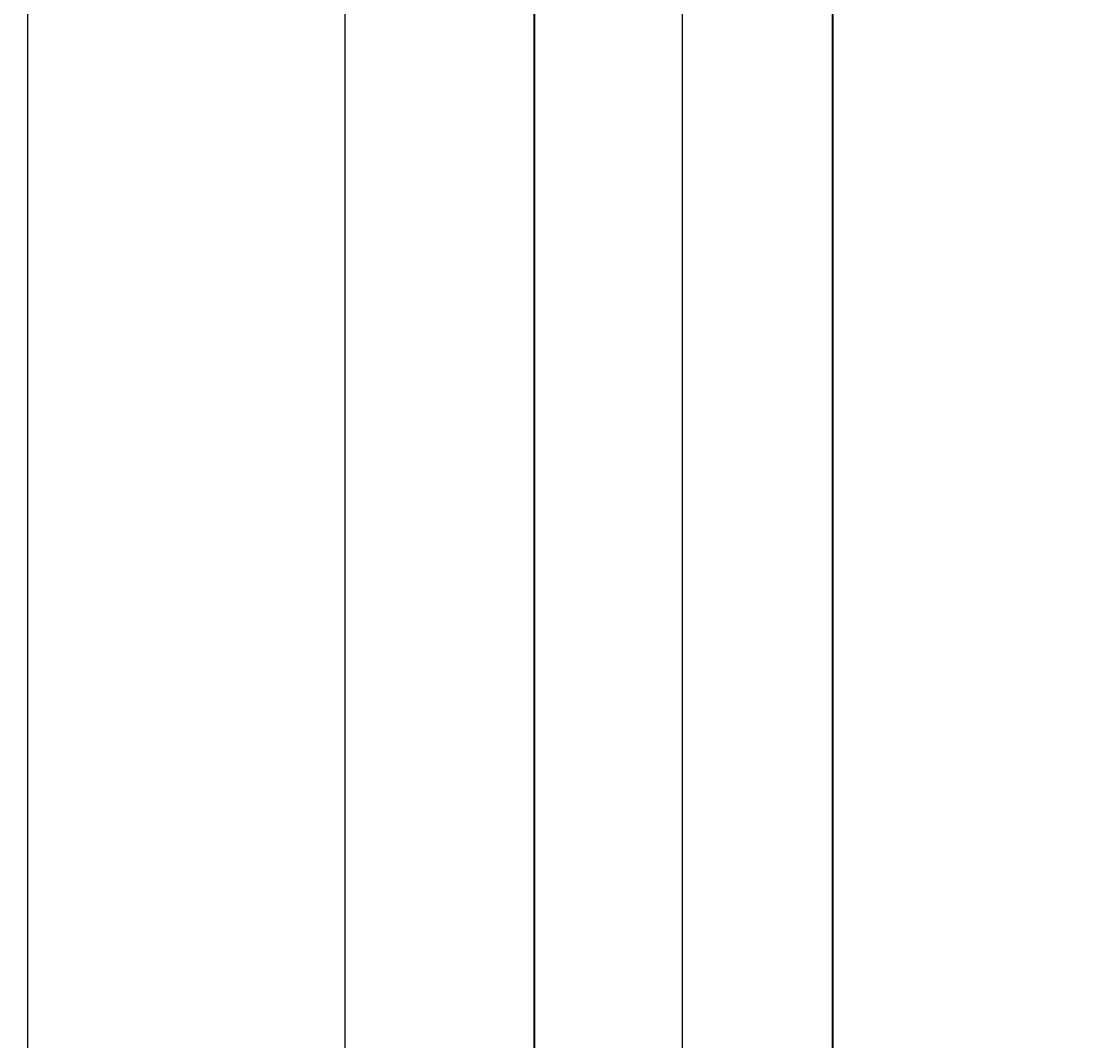
# Model space of a CAD drawing. Units: inches. Extents: x -6 to 289, y -8 to 323.
# Tile 43 of 107: x -6 to 46, y 223 to 273. Entities that reach past the tile are written whole.
import ezdxf

# ---------------------------------------------------------------- set-up
doc = ezdxf.new("R2010")
doc.units = ezdxf.units.IN
doc.header["$MEASUREMENT"] = 0
doc.layers.add('A-ANNO-DIMS', color=2, linetype='Continuous', lineweight=18)
doc.layers.add('A-ELEV', color=7, linetype='Continuous', lineweight=35)
doc.styles.get("Standard").update_dxf_attribs({"font": 'arial.ttf'})
doc.dimstyles.get("Standard").update_dxf_attribs({"dimtxt": 0.18, "dimasz": 0.18, "dimexe": 0.18, "dimexo": 0.0625, "dimgap": 0.09, "dimtad": 0, "dimtih": 1, "dimtoh": 1, "dimdec": 4, "dimzin": 0, "dimdsep": 46, "dimtxsty": 'Standard', "dimcen": 0.09, "dimadec": 0, "dimazin": 0, "dimtfac": 1, "dimtdec": 4, "dimtofl": 0, "dimtmove": 0, "dimatfit": 3, "dimfxl": 1, "dimtolj": 1, "dimtzin": 0, "dimarcsym": 0})

# ---------------------------------------------------------------- blocks, each defined once
blk = doc.blocks.new('*D19')
at = {"layer": 'A-ANNO-DIMS', "color": 0, "lineweight": -2, "transparency": 16777216}
for p, q in [((45.681, 277.043), (-5.737, 277.043)), ((-5.557, 276.863), (-5.557, 179.825)), ((-5.557, 82.423), (-5.557, 179.461)), ((45.681, 82.243), (-5.737, 82.243))]:
    blk.add_line(p, q, dxfattribs=at)
at = {"layer": 'A-ANNO-DIMS', "color": 0, "transparency": 16777216}
for points in [[(-5.587, 276.863), (-5.527, 276.863), (-5.557, 277.043)], [(-5.587, 82.423), (-5.527, 82.423), (-5.557, 82.243)]]:
    blk.add_solid(points, dxfattribs=at)
at = {"layer": 'Defpoints', "color": 0, "transparency": 16777216}
for p in [(-5.557, 277.043), (45.744, 277.043), (45.744, 82.243)]:
    blk.add_point(p, dxfattribs=at)
at = {"layer": 'A-ANNO-DIMS', "color": 0, "transparency": 16777216, "insert": (-5.557, 179.643), "char_height": 0.18, "attachment_point": 5}
blk.add_mtext('\\A1;194.8', dxfattribs=at)
blk = doc.blocks.new('*D22')
at = {"layer": 'A-ANNO-DIMS', "color": 0, "lineweight": -2, "transparency": 16777216}
for p, q in [((19.101, 307.289), (-5.737, 307.289)), ((-5.557, 307.109), (-5.557, 157.471)), ((-5.557, 7.469), (-5.557, 157.107)), ((11.907, 7.289), (-5.737, 7.289))]:
    blk.add_line(p, q, dxfattribs=at)
at = {"layer": 'A-ANNO-DIMS', "color": 0, "transparency": 16777216}
for points in [[(-5.587, 307.109), (-5.527, 307.109), (-5.557, 307.289)], [(-5.587, 7.469), (-5.527, 7.469), (-5.557, 7.289)]]:
    blk.add_solid(points, dxfattribs=at)
at = {"layer": 'Defpoints', "color": 0, "transparency": 16777216}
for p in [(19.164, 307.289), (-5.557, 7.289), (11.969, 7.289)]:
    blk.add_point(p, dxfattribs=at)
at = {"layer": 'A-ANNO-DIMS', "color": 0, "transparency": 16777216, "insert": (-5.557, 157.289), "char_height": 0.18, "attachment_point": 5}
blk.add_mtext('\\A1;300', dxfattribs=at)
blk = doc.blocks.new('*D27')
at = {"layer": 'A-ANNO-DIMS', "color": 0, "lineweight": -2, "transparency": 16777216}
for p, q in [((19.226, 307.289), (288.653, 307.289)), ((288.473, 307.109), (288.473, 277.471)), ((288.473, 247.469), (288.473, 277.107)), ((247.226, 247.289), (288.653, 247.289))]:
    blk.add_line(p, q, dxfattribs=at)
at = {"layer": 'A-ANNO-DIMS', "color": 0, "transparency": 16777216}
for points in [[(288.443, 307.109), (288.503, 307.109), (288.473, 307.289)], [(288.443, 247.469), (288.503, 247.469), (288.473, 247.289)]]:
    blk.add_solid(points, dxfattribs=at)
at = {"layer": 'Defpoints', "color": 0, "transparency": 16777216}
for p in [(19.164, 307.289), (288.473, 307.289), (247.164, 247.289)]:
    blk.add_point(p, dxfattribs=at)
at = {"layer": 'A-ANNO-DIMS', "color": 0, "transparency": 16777216, "insert": (288.473, 277.289), "char_height": 0.18, "attachment_point": 5}
blk.add_mtext('\\A1;60', dxfattribs=at)
blk = doc.blocks.new('*D57')
at = {"layer": 'A-ANNO-DIMS', "color": 0, "lineweight": -2, "transparency": 16777216}
for p, q in [((9.943, 68.495), (9.943, 322.969)), ((10.123, 322.789), (17.788, 322.789)), ((26.223, 322.789), (18.558, 322.789)), ((26.403, 68.495), (26.403, 322.969))]:
    blk.add_line(p, q, dxfattribs=at)
at = {"layer": 'A-ANNO-DIMS', "color": 0, "transparency": 16777216}
for points in [[(10.123, 322.819), (10.123, 322.759), (9.943, 322.789)], [(26.223, 322.819), (26.223, 322.759), (26.403, 322.789)]]:
    blk.add_solid(points, dxfattribs=at)
at = {"layer": 'Defpoints', "color": 0, "transparency": 16777216}
for p in [(26.403, 322.789), (9.943, 68.432), (26.403, 68.432)]:
    blk.add_point(p, dxfattribs=at)
at = {"layer": 'A-ANNO-DIMS', "color": 0, "transparency": 16777216, "insert": (18.173, 322.789), "char_height": 0.18, "attachment_point": 5}
blk.add_mtext('\\A1;16.46', dxfattribs=at)

msp = doc.modelspace()

# ---------------------------------------------------------------- linework, layer by layer
at = {"layer": 'A-ELEV'}
msp.add_line((19.1638, 307.2888), (19.1638, 68.4322), dxfattribs=at)
msp.add_lwpolyline([(33.7437, 289.0427), (99.7007, 289.0427), (99.7007, 70.2425), (33.7437, 70.2425)], close=True, dxfattribs=at)

# ---------------------------------------------------------------- dimensions: what is measured, and where the dimension line sits
at = {"layer": 'A-ANNO-DIMS'}
dim = msp.add_linear_dim(base=(26.403, 322.7888), p1=(9.943, 68.4322), p2=(26.403, 68.4322), dimstyle='Standard', override={"dimdec": 2, "dimlfac": 1, "dimrnd": 0, "dimzin": 0, "dimdsep": 46, "dimlunit": 2}, dxfattribs=at)
dim.commit()
dim.dimension.update_dxf_attribs({"geometry": '*D57', "text_midpoint": (18.173, 322.7888)})
for base, p1, p2, override, picture, middle in [((-5.557, 7.2888), (19.1638, 307.2888), (11.9692, 7.2888), {"dimdec": 0, "dimlfac": 1, "dimrnd": 0, "dimzin": 0, "dimdsep": 46, "dimlunit": 2}, '*D22', (-5.557, 157.2888)), ((288.4733, 307.2888), (247.1638, 247.2888), (19.1638, 307.2888), {"dimdec": 0, "dimlfac": 1, "dimrnd": 0, "dimzin": 0, "dimdsep": 46, "dimlunit": 2}, '*D27', (288.4733, 277.2888)), ((-5.557, 277.0427), (45.7437, 82.2425), (45.7437, 277.0427), {"dimdec": 1, "dimlfac": 1, "dimrnd": 0, "dimzin": 0, "dimdsep": 46, "dimlunit": 2}, '*D19', (-5.557, 179.6426))]:
    dim = msp.add_linear_dim(base=base, p1=p1, p2=p2, angle=90, dimstyle='Standard', override=override, dxfattribs=at)
    dim.commit()
    dim.dimension.update_dxf_attribs({"geometry": picture, "text_midpoint": middle})

doc.saveas('drawing.dxf')
